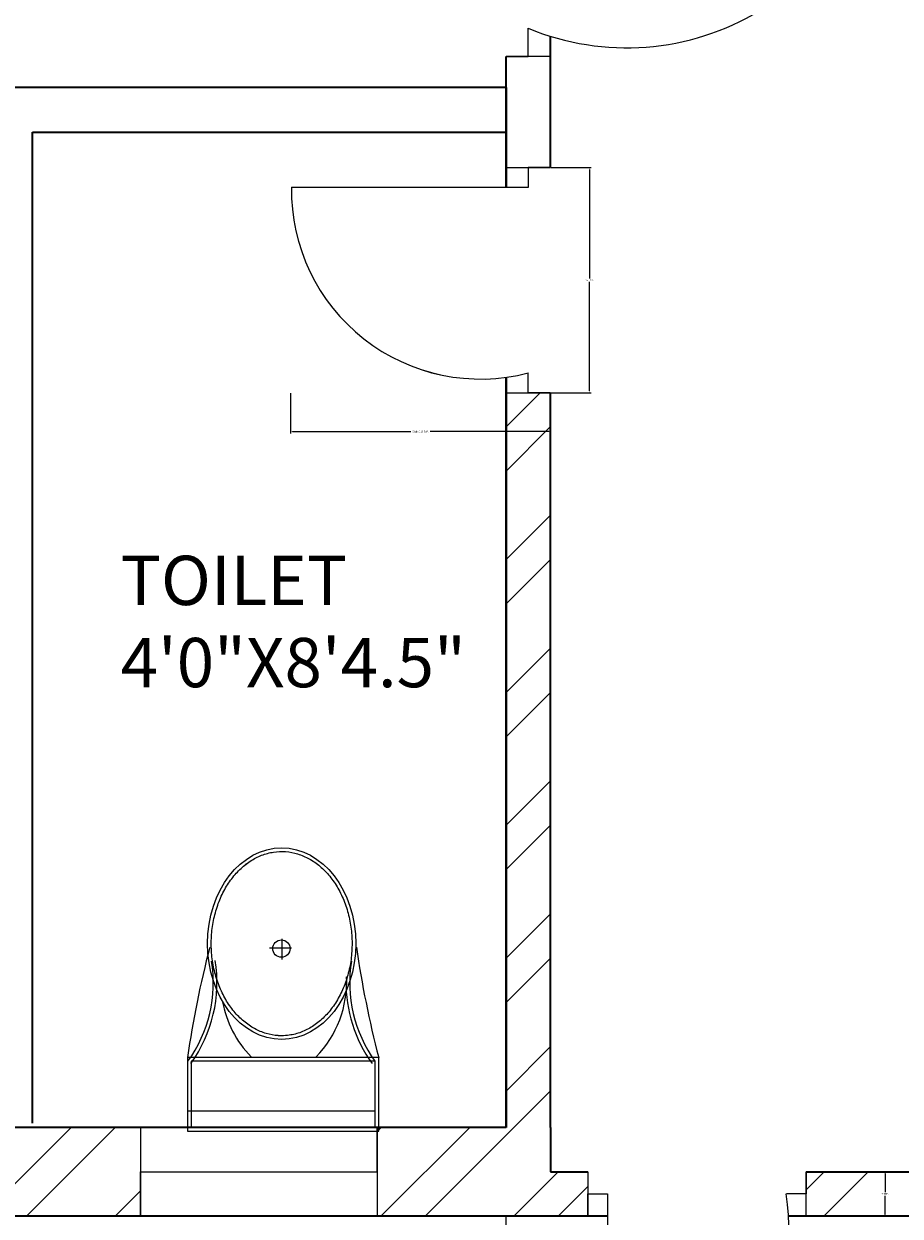
# Model space of a CAD drawing. Units: inches. Extents: x 2120 to 4013, y 1390 to 3019.
# Tile 10 of 59: x 2448 to 2537, y 1582 to 1702. Entities that reach past the tile are written whole.
import ezdxf

# ---------------------------------------------------------------- set-up
doc = ezdxf.new("R2010")
doc.units = ezdxf.units.IN
for name, color, linetype, lineweight in [('A-ANNO-DIMS', 2, 'Continuous', 18), ('A-AREA-IDEN', 7, 'Continuous', 18), ('A-DOOR', 3, 'Continuous', 18), ('A-FLOR-DECK', 7, 'Continuous', 25), ('A-FLOR-FIXT', 9, 'Continuous', 18), ('A-GLAZ', 4, 'Continuous', 18), ('A-WALL', 7, 'Continuous', 35), ('A-WALL-PATT', 252, 'Continuous', 13)]:
    doc.layers.add(name, color=color, linetype=linetype, lineweight=lineweight)
doc.styles.get("Standard").update_dxf_attribs({"font": 'arial.ttf'})
doc.dimstyles.get("Standard").update_dxf_attribs({"dimtxt": 0.18, "dimasz": 0.18, "dimexe": 0.18, "dimexo": 0.0625, "dimgap": 0.09, "dimtad": 0, "dimtih": 1, "dimtoh": 1, "dimdec": 4, "dimzin": 0, "dimdsep": 46, "dimtxsty": 'Standard', "dimcen": 0.09, "dimadec": 0, "dimazin": 0, "dimtfac": 1, "dimtdec": 4, "dimtofl": 0, "dimtmove": 0, "dimatfit": 3, "dimfxl": 1, "dimtolj": 1, "dimtzin": 0, "dimarcsym": 0})

# ---------------------------------------------------------------- blocks, each defined once
blk = doc.blocks.new('A$C31115884')
for p, q in [((257.5, 466.4), (257.5, 523.2)), ((283.1, 497.7), (223.4, 497.7)), ((0, 200), (0, 0)), ((520, 200), (0, 200)), ((520, 0), (520, 200)), ((10, 190), (10, 10)), ((510, 190), (10, 190)), ((510, 10), (510, 190)), ((510, 54.5), (0, 54.5)), ((10, 10), (510, 10)), ((0, 0), (520, 0))]:
    blk.add_line(p, q)
blk.add_circle((255.6, 496.4), 23.6)
for centre, radius, start, end in [((2777.7, -204.6), 2807, 165.4549, 171.7133), ((3237, 905), 2807, 188.2867, 194.5451), ((-294.5, 403.3), 364.7, 324.2091, 9.3499), ((-294.5, 403.3), 374.7, 324.2091, 9.3499), ((805.8, 403.3), 364.7, 170.6501, 215.7909), ((139.5, 406.2), 293.5, 315.8436, 2.6563), ((805.8, 403.3), 374.7, 179.2036, 215.7909), ((383.6, 406.2), 293.5, 190.2774, 224.1564)]:
    blk.add_arc(centre, radius, start, end)
blk.add_ellipse((256.2, 509.9), major_axis=(0, -260.7), ratio=0.772727)
blk.add_open_spline([(256.2, 259.2), (263.1, 259.2), (270, 259.7), (287.8, 262.3), (298.7, 265.1), (319.9, 273.1), (330.2, 278.4), (350.1, 291.1), (359.7, 298.7), (377.7, 315.9), (386.2, 325.5), (401.7, 346.6), (408.8, 358.1), (421.3, 382.5), (426.8, 395.5), (435.9, 422.4), (439.5, 436.4), (444.8, 465.1), (446.5, 479.7), (447.9, 509.2), (447.6, 524), (445, 553.3), (442.7, 567.8), (436.3, 596), (432.1, 609.7), (421.9, 636), (416, 648.6), (402.5, 672.1), (395, 683), (378.6, 703), (369.8, 712.1), (351.1, 728), (341.3, 734.8), (320.9, 746.2), (310.4, 750.7), (288.9, 757.3), (278, 759.4), (256, 761), (245, 760.6), (223.1, 757.2), (212.3, 754.3), (191.1, 746.1), (180.8, 740.7), (160.9, 727.8), (151.4, 720.1), (133.5, 702.7), (125.1, 693), (109.6, 671.7), (102.6, 660.2), (90.2, 635.7), (84.9, 622.7), (76, 595.6), (72.4, 581.6), (67.2, 552.9), (65.6, 538.2), (64.4, 508.8), (64.8, 494), (67.5, 464.7), (69.9, 450.2), (76.6, 422), (80.8, 408.3), (91.1, 382.2), (97.2, 369.7), (110.8, 346.3), (118.4, 335.4), (134.8, 315.6), (143.7, 306.7), (162.4, 290.9), (172.3, 284.2), (192.8, 273), (203.3, 268.6), (224.8, 262.2), (235.8, 260.2), (249.9, 259.3), (253, 259.2), (256.2, 259.2)], degree=3, knots=[0, 0, 0, 0, 0.110105, 0.110105, 0.285049, 0.285049, 0.459994, 0.459994, 0.634938, 0.634938, 0.809882, 0.809882, 0.984827, 0.984827, 1.159771, 1.159771, 1.334715, 1.334715, 1.50966, 1.50966, 1.684604, 1.684604, 1.859549, 1.859549, 2.034493, 2.034493, 2.209437, 2.209437, 2.384382, 2.384382, 2.559326, 2.559326, 2.73427, 2.73427, 2.909215, 2.909215, 3.084159, 3.084159, 3.259103, 3.259103, 3.434048, 3.434048, 3.608992, 3.608992, 3.783936, 3.783936, 3.958881, 3.958881, 4.133825, 4.133825, 4.30877, 4.30877, 4.483714, 4.483714, 4.658658, 4.658658, 4.833603, 4.833603, 5.008547, 5.008547, 5.183491, 5.183491, 5.358436, 5.358436, 5.53338, 5.53338, 5.708324, 5.708324, 5.883269, 5.883269, 6.058213, 6.058213, 6.233158, 6.233158, 6.283185, 6.283185, 6.283185, 6.283185])
blk = doc.blocks.new('DOOR-SWING-24IN-91p57DEG')
for p, q in [((0, 26.25), (0, 21.75)), ((22.12, 21.75), (22.12, 26.25)), ((22.12, 26.25), (22.12, 24)), ((0, 21.75), (0, 24)), ((0, 24), (2, 24)), ((2, 24), (2, 0)), ((22.12, 24), (20.12, 24))]:
    blk.add_line(p, q)
blk.add_arc((-0.62, 20.81), 20.98, 277.1643, 8.7385)
blk = doc.blocks.new('DOOR-SWING-24IN-105p55DEG')
for p, q in [((21.75, 22.82), (26.25, 22.82)), ((26.25, 22.82), (24, 22.82)), ((24, 22.82), (24, 20.82)), ((24, 20.82), (0, 20.82)), ((24, 0), (24, 2)), ((21.75, 0), (26.25, 0)), ((26.25, 0), (24, 0))]:
    blk.add_line(p, q)
blk.add_arc((19.15, 20.53), 19.15, 179.1207, 284.6739)
blk = doc.blocks.new('DOOR-SWING-36IN-107p00DEG')
for p, q in [((4.5, 26.58), (0, 26.58)), ((0, 26.58), (2.25, 26.58)), ((2.25, 26.58), (2.25, 24.58)), ((2.25, 24.58), (38.25, 24.58)), ((2.25, 0), (2.25, 2.87)), ((4.5, 0), (0, 0)), ((0, 0), (2.25, 0))]:
    blk.add_line(p, q)
blk.add_arc((12.22, 27.04), 26.15, 247.599, 354.5999)
blk = doc.blocks.new('WIN-PLAN-24IN-03')
for p, q in [((9, 24), (0, 24)), ((0, 24), (4.5, 24)), ((4.5, 24), (4.5, 0)), ((9, 0), (0, 0)), ((4.5, 0), (9, 0))]:
    blk.add_line(p, q)
blk = doc.blocks.new('*D137')
at = {"layer": 'A-ANNO-DIMS', "color": 0, "lineweight": -2, "transparency": 16777216}
for p, q in [((2474.89, 1664.96), (2474.89, 1660.89)), ((2501.23, 1664.96), (2501.23, 1660.89)), ((2475.07, 1661.07), (2487.07, 1661.07)), ((2501.05, 1661.07), (2489.05, 1661.07))]:
    blk.add_line(p, q, dxfattribs=at)
at = {"layer": 'A-ANNO-DIMS', "color": 0, "transparency": 16777216}
for points in [[(2475.07, 1661.1), (2475.07, 1661.04), (2474.89, 1661.07)], [(2501.05, 1661.1), (2501.05, 1661.04), (2501.23, 1661.07)]]:
    blk.add_solid(points, dxfattribs=at)
at = {"layer": 'Defpoints', "color": 0, "transparency": 16777216}
for p in [(2474.89, 1665.02), (2501.23, 1665.02), (2501.23, 1661.07)]:
    blk.add_point(p, dxfattribs=at)
at = {"layer": 'A-ANNO-DIMS', "color": 0, "transparency": 16777216, "insert": (2488.06, 1661.07), "char_height": 0.18, "attachment_point": 5}
blk.add_mtext('\\A1;SWING 26 TYP.', dxfattribs=at)
blk = doc.blocks.new('*D138')
at = {"layer": 'A-ANNO-DIMS', "color": 0, "lineweight": -2, "transparency": 16777216}
for p, q in [((2501.3, 1687.84), (2505.36, 1687.84)), ((2505.18, 1687.66), (2505.18, 1676.61)), ((2505.18, 1665.2), (2505.18, 1676.25)), ((2501.3, 1665.02), (2505.36, 1665.02))]:
    blk.add_line(p, q, dxfattribs=at)
at = {"layer": 'A-ANNO-DIMS', "color": 0, "transparency": 16777216}
for points in [[(2505.15, 1687.66), (2505.21, 1687.66), (2505.18, 1687.84)], [(2505.15, 1665.2), (2505.21, 1665.2), (2505.18, 1665.02)]]:
    blk.add_solid(points, dxfattribs=at)
at = {"layer": 'Defpoints', "color": 0, "transparency": 16777216}
for p in [(2501.23, 1687.84), (2505.18, 1687.84), (2501.23, 1665.02)]:
    blk.add_point(p, dxfattribs=at)
at = {"layer": 'A-ANNO-DIMS', "color": 0, "transparency": 16777216, "insert": (2505.18, 1676.43), "char_height": 0.18, "attachment_point": 5}
blk.add_mtext('\\A1;23 TYP.', dxfattribs=at)
blk = doc.blocks.new('*D192')
at = {"layer": 'A-ANNO-DIMS', "color": 0, "lineweight": -2, "transparency": 16777216}
for p, q in [((2544.07, 1586.03), (2534.96, 1586.03)), ((2535.14, 1585.85), (2535.14, 1583.96)), ((2535.14, 1581.71), (2535.14, 1583.6)), ((2544.07, 1581.53), (2534.96, 1581.53))]:
    blk.add_line(p, q, dxfattribs=at)
at = {"layer": 'A-ANNO-DIMS', "color": 0, "transparency": 16777216}
for points in [[(2535.11, 1585.85), (2535.17, 1585.85), (2535.14, 1586.03)], [(2535.11, 1581.71), (2535.17, 1581.71), (2535.14, 1581.53)]]:
    blk.add_solid(points, dxfattribs=at)
at = {"layer": 'Defpoints', "color": 0, "transparency": 16777216}
for p in [(2535.14, 1586.03), (2544.14, 1586.03), (2544.14, 1581.53)]:
    blk.add_point(p, dxfattribs=at)
at = {"layer": 'A-ANNO-DIMS', "color": 0, "transparency": 16777216, "insert": (2535.14, 1583.78), "char_height": 0.18, "attachment_point": 5}
blk.add_mtext('\\A1;5 TYP.', dxfattribs=at)

msp = doc.modelspace()

# ---------------------------------------------------------------- hatches: boundary and pattern name
at = {"layer": 'A-WALL-PATT'}
h = msp.add_hatch(dxfattribs=at)
h.set_pattern_fill('ANSI32', color=256)
h.paths.add_polyline_path([(2271.7331, 2343.531), (2283.3788, 2343.531), (2283.3788, 2348.031), (2283.3788, 2352.5306), (2262.7331, 2352.5306), (2262.7331, 2182.638), (2267.2331, 2182.638), (2271.7331, 2182.638), (2271.7331, 2219.031), (2391.7331, 2219.031), (2391.7331, 2214.189), (2393.9831, 2214.189), (2396.2331, 2214.189), (2396.2331, 2219.031), (2420.2331, 2219.031), (2420.2331, 2225.7535), (2417.2197, 2225.7535), (2415.7331, 2225.7535), (2415.7331, 2223.5306), (2271.7331, 2223.5306)])
h.paths.add_polyline_path([(2380.0942, 2352.5306), (2343.3788, 2352.5306), (2343.3788, 2343.531), (2363.2331, 2343.531), (2363.2331, 2288.8489), (2365.4831, 2288.8489), (2367.7331, 2288.8489), (2367.7331, 2343.531), (2380.0942, 2343.531)], flags=17)
h.paths.add_polyline_path([(2432.4339, 2352.5306), (2404.0943, 2352.5306), (2404.0943, 2343.531), (2415.7331, 2343.531), (2415.7331, 2264.0306), (2367.7331, 2264.0306), (2367.7331, 2266.4872), (2363.2331, 2266.4872), (2363.2331, 2259.531), (2367.7331, 2259.531), (2415.7331, 2259.531), (2415.7331, 2255.0658), (2420.2331, 2255.0658), (2420.2331, 2259.531), (2424.5717, 2259.531), (2424.5717, 2261.781), (2424.5717, 2264.0306), (2420.2331, 2264.0306), (2420.2331, 2343.531), (2432.4339, 2343.531)])
h.paths.add_polyline_path([(2508.9115, 2352.5306), (2456.4339, 2352.5306), (2456.4339, 2343.531), (2468.2331, 2343.531), (2468.2331, 2264.0306), (2448.0487, 2264.0306), (2448.0487, 2259.531), (2468.2331, 2259.531), (2468.2331, 2255.5496), (2472.7331, 2255.5496), (2472.7331, 2343.531), (2508.9115, 2343.531)])
h.paths.add_polyline_path([(2637.7331, 2352.5306), (2544.9116, 2352.5306), (2544.9116, 2343.531), (2589.7331, 2343.531), (2633.2331, 2343.531), (2637.7331, 2343.531)])
h.paths.add_polyline_path([(2594.2331, 2343.5306), (2589.7331, 2343.5306), (2589.7331, 2259.5306), (2589.7331, 2252.4915), (2591.9831, 2252.4915), (2594.2331, 2252.4915)])
h.paths.add_polyline_path([(2637.7331, 2223.5306), (2594.2331, 2223.5306), (2594.2331, 2230.1988), (2591.9831, 2230.1988), (2589.7331, 2230.1988), (2589.7331, 2223.5306), (2472.7331, 2223.5306), (2468.2331, 2223.5306), (2468.2331, 2219.031), (2628.7331, 2219.031), (2628.7331, 2138.031), (2637.7331, 2138.031)])
h.paths.add_polyline_path([(3822.6535, 2458.4402), (3874.9468, 2458.4402), (3874.9468, 2476.9866), (3822.6535, 2476.9866)], flags=9)
h.paths.add_polyline_path([(3834.6921, 2781.8174), (3935.9206, 2781.8174), (3935.9206, 2800.3638), (3834.6921, 2800.3638)], flags=9)
h.paths.add_polyline_path([(3832.2843, 2837.9683), (3884.5776, 2837.9683), (3884.5776, 2856.5146), (3832.2843, 2856.5146)], flags=9)
h.paths.add_polyline_path([(3830.9388, 2861.4782), (3956.8958, 2861.4782), (3956.8958, 2880.0245), (3830.9388, 2880.0245)], flags=9)
h.paths.add_polyline_path([(3870.6966, 2352.5752), (3887.9272, 2352.5752), (3887.9272, 2377.3037), (3870.6966, 2377.3037)], flags=9)
h.paths.add_polyline_path([(3289.2701, 2413.161), (3435.2223, 2413.161), (3435.2223, 2450.2538), (3289.2701, 2450.2538)], flags=9)
h.paths.add_polyline_path([(2487.6944, 2414.3601), (2637.8335, 2414.3601), (2637.8335, 2451.4528), (2487.6944, 2451.4528)], flags=9)
h.paths.add_polyline_path([(2567.3724, 1457.9199), (2815.296, 1457.9199), (2815.296, 1495.0127), (2567.3724, 1495.0127)], flags=9)
h.paths.add_polyline_path([(2655.3825, 2093.2363), (2685.9555, 2093.2363), (2685.9555, 2111.8937), (2655.3825, 2111.8937)], flags=9)
h.paths.add_polyline_path([(2543.9218, 1550.6671), (2587.8406, 1550.6671), (2587.8406, 1569.3244), (2543.9218, 1569.3244)], flags=9)
h.paths.add_polyline_path([(2905.1384, 1543.8113), (2949.0572, 1543.8113), (2949.0572, 1562.4686), (2905.1384, 1562.4686)], flags=9)
h.paths.add_polyline_path([(2736.4118, 1702.4736), (2784.2153, 1702.4736), (2784.2153, 1721.1309), (2736.4118, 1721.1309)], flags=9)
h.paths.add_polyline_path([(2912.8666, 1710.4168), (2951.707, 1710.4168), (2951.707, 1729.0741), (2912.8666, 1729.0741)], flags=9)
h.paths.add_polyline_path([(2923.5785, 1763.5038), (2959.7279, 1763.5038), (2959.7279, 1782.1611), (2923.5785, 1782.1611)], flags=9)
h.paths.add_polyline_path([(2925.2114, 1809.6137), (2967.1861, 1809.6137), (2967.1861, 1828.271), (2925.2114, 1828.271)], flags=9)
h.paths.add_polyline_path([(2996.2711, 1878.9003), (2996.2711, 1913.109), (2977.6138, 1913.109), (2977.6138, 1878.9003)], flags=9)
h.paths.add_polyline_path([(2883.0859, 1895.7192), (2927.1855, 1895.7192), (2927.1855, 1914.3766), (2883.0859, 1914.3766)], flags=9)
h.paths.add_polyline_path([(2787.3924, 1810.8013), (2841.0213, 1810.8013), (2841.0213, 1829.4587), (2787.3924, 1829.4587)], flags=9)
h.paths.add_polyline_path([(2775.6399, 2101.7395), (2829.2689, 2101.7395), (2829.2689, 2120.3968), (2775.6399, 2120.3968)], flags=9)
h.paths.add_polyline_path([(2913.0263, 2075.817), (2951.8667, 2075.817), (2951.8667, 2094.4744), (2913.0263, 2094.4744)], flags=9)
h.paths.add_polyline_path([(2929.966, 2133.3669), (2966.1154, 2133.3669), (2966.1154, 2152.0243), (2929.966, 2152.0243)], flags=9)
h.paths.add_polyline_path([(2932.7502, 2182.6088), (2968.8996, 2182.6088), (2968.8996, 2201.2662), (2932.7502, 2201.2662)], flags=9)
h.paths.add_polyline_path([(2996.0681, 2266.3173), (2996.0681, 2300.5261), (2977.4108, 2300.5261), (2977.4108, 2266.3173)], flags=9)
h.paths.add_polyline_path([(2885.1039, 2279.2186), (2929.2035, 2279.2186), (2929.2035, 2297.8759), (2885.1039, 2297.8759)], flags=9)
h.paths.add_polyline_path([(2735.7042, 2218.3197), (2783.5078, 2218.3197), (2783.5078, 2236.9771), (2735.7042, 2236.9771)], flags=9)
h.paths.add_polyline_path([(2635.6049, 2044.0085), (2648.9678, 2044.0085), (2648.9678, 2054.312), (2635.6049, 2054.312)], flags=9)
h.paths.add_polyline_path([(2714.0148, 1923.0473), (2727.3777, 1923.0473), (2727.3777, 1933.3508), (2714.0148, 1933.3508)], flags=9)
h.paths.add_polyline_path([(2709.0345, 1988.1628), (2722.3974, 1988.1628), (2722.3974, 1998.4663), (2709.0345, 1998.4663)], flags=9)
h.paths.add_polyline_path([(2592.8935, 1962.1763), (2606.2564, 1962.1763), (2606.2564, 1972.4799), (2592.8935, 1972.4799)], flags=9)
h.paths.add_polyline_path([(2618.3996, 1985.9724), (2644.1942, 1985.9724), (2644.1942, 1996.2759), (2618.3996, 1996.2759)], flags=9)
h.paths.add_polyline_path([(2601.279, 1920.5869), (2614.6419, 1920.5869), (2614.6419, 1930.8904), (2601.279, 1930.8904)], flags=9)
h.paths.add_polyline_path([(2692.3278, 1932.7645), (2704.5311, 1932.7645), (2704.5311, 1943.0681), (2692.3278, 1943.0681)], flags=9)
h.paths.add_polyline_path([(2311.122, 1672.7318), (2355.0408, 1672.7318), (2355.0408, 1691.3892), (2311.122, 1691.3892)], flags=9)
h.paths.add_polyline_path([(2456.2551, 1632.3198), (2492.4796, 1632.3198), (2492.4796, 1650.9772), (2456.2551, 1650.9772)], flags=9)
h.paths.add_polyline_path([(2401.0766, 1631.4793), (2437.301, 1631.4793), (2437.301, 1650.1367), (2401.0766, 1650.1367)], flags=9)
h.paths.add_polyline_path([(2546.7054, 1700.9235), (2594.509, 1700.9235), (2594.509, 1719.5809), (2546.7054, 1719.5809)], flags=9)
h.paths.add_polyline_path([(2445.4866, 1766.9937), (2497.5261, 1766.9937), (2497.5261, 1785.651), (2445.4866, 1785.651)], flags=9)
h.paths.add_polyline_path([(2287.9992, 1739.7675), (2326.8396, 1739.7675), (2326.8396, 1758.4248), (2287.9992, 1758.4248)], flags=9)
h.paths.add_polyline_path([(2458.5279, 1924.7607), (2510.5675, 1924.7607), (2510.5675, 1943.4181), (2458.5279, 1943.4181)], flags=9)
h.paths.add_polyline_path([(2309.2811, 1902.7642), (2345.4305, 1902.7642), (2345.4305, 1921.4215), (2309.2811, 1921.4215)], flags=9)
h.paths.add_polyline_path([(2490.7554, 2018.9392), (2530.7896, 2018.9392), (2530.7896, 2037.5965), (2490.7554, 2037.5965)], flags=9)
h.paths.add_polyline_path([(2402.143, 2024.7393), (2438.5414, 2024.7393), (2438.5414, 2043.3966), (2402.143, 2043.3966)], flags=9)
h.paths.add_polyline_path([(2287.856, 1931.7926), (2326.6964, 1931.7926), (2326.6964, 1950.4499), (2287.856, 1950.4499)], flags=9)
h.paths.add_polyline_path([(2281.7979, 2193.5771), (2320.6383, 2193.5771), (2320.6383, 2212.2344), (2281.7979, 2212.2344)], flags=25)
h.paths.add_polyline_path([(2484.0754, 2093.892), (2536.115, 2093.892), (2536.115, 2112.5494), (2484.0754, 2112.5494)], flags=9)
h.paths.add_polyline_path([(2624.7948, 2281.8639), (2624.7948, 2311.4137), (2606.1375, 2311.4137), (2606.1375, 2281.8639)], flags=9)
h.paths.add_polyline_path([(2507.5036, 2290.3639), (2541.934, 2290.3639), (2541.934, 2309.0212), (2507.5036, 2309.0212)], flags=9)
h.paths.add_polyline_path([(2423.1076, 2285.2202), (2459.332, 2285.2202), (2459.332, 2303.8776), (2423.1076, 2303.8776)], flags=9)
h.paths.add_polyline_path([(2374.5467, 2289.6272), (2410.7711, 2289.6272), (2410.7711, 2308.2846), (2374.5467, 2308.2846)], flags=25)
h.paths.add_polyline_path([(2277.4907, 2227.5651), (2316.3311, 2227.5651), (2316.3311, 2246.2224), (2277.4907, 2246.2224)], flags=25)
h.paths.add_polyline_path([(2655.3825, 2093.2367), (2685.9555, 2093.2367), (2685.9555, 2111.894), (2655.3825, 2111.894)], flags=9)
h.paths.add_polyline_path([(2543.9217, 1550.6674), (2587.8406, 1550.6674), (2587.8406, 1569.3247), (2543.9217, 1569.3247)], flags=9)
h.paths.add_polyline_path([(2905.1384, 1543.8116), (2949.0572, 1543.8116), (2949.0572, 1562.4689), (2905.1384, 1562.4689)], flags=9)
h.paths.add_polyline_path([(2736.4118, 1702.4739), (2784.2153, 1702.4739), (2784.2153, 1721.1312), (2736.4118, 1721.1312)], flags=9)
h.paths.add_polyline_path([(2912.8666, 1710.4171), (2951.707, 1710.4171), (2951.707, 1729.0744), (2912.8666, 1729.0744)], flags=9)
h.paths.add_polyline_path([(2923.5785, 1763.5041), (2959.7279, 1763.5041), (2959.7279, 1782.1614), (2923.5785, 1782.1614)], flags=9)
h.paths.add_polyline_path([(2925.2114, 1809.614), (2967.1861, 1809.614), (2967.1861, 1828.2713), (2925.2114, 1828.2713)], flags=9)
h.paths.add_polyline_path([(2996.2711, 1878.9006), (2996.2711, 1913.1094), (2977.6137, 1913.1094), (2977.6137, 1878.9006)], flags=9)
h.paths.add_polyline_path([(2883.0859, 1895.7195), (2927.1855, 1895.7195), (2927.1855, 1914.3769), (2883.0859, 1914.3769)], flags=9)
h.paths.add_polyline_path([(2787.3924, 1810.8016), (2841.0213, 1810.8016), (2841.0213, 1829.459), (2787.3924, 1829.459)], flags=9)
h.paths.add_polyline_path([(2775.6399, 2101.7398), (2829.2688, 2101.7398), (2829.2688, 2120.3971), (2775.6399, 2120.3971)], flags=9)
h.paths.add_polyline_path([(2913.0263, 2075.8173), (2951.8667, 2075.8173), (2951.8667, 2094.4747), (2913.0263, 2094.4747)], flags=9)
h.paths.add_polyline_path([(2929.966, 2133.3672), (2966.1154, 2133.3672), (2966.1154, 2152.0246), (2929.966, 2152.0246)], flags=9)
h.paths.add_polyline_path([(2932.7502, 2182.6091), (2968.8996, 2182.6091), (2968.8996, 2201.2665), (2932.7502, 2201.2665)], flags=9)
h.paths.add_polyline_path([(2996.0681, 2266.3176), (2996.0681, 2300.5264), (2977.4108, 2300.5264), (2977.4108, 2266.3176)], flags=9)
h.paths.add_polyline_path([(2885.1039, 2279.2189), (2929.2035, 2279.2189), (2929.2035, 2297.8762), (2885.1039, 2297.8762)], flags=9)
h.paths.add_polyline_path([(2735.7042, 2218.32), (2783.5078, 2218.32), (2783.5078, 2236.9774), (2735.7042, 2236.9774)], flags=9)
h.paths.add_polyline_path([(2635.6048, 2044.0088), (2648.9677, 2044.0088), (2648.9677, 2054.3123), (2635.6048, 2054.3123)], flags=9)
h.paths.add_polyline_path([(2714.0148, 1923.0476), (2727.3777, 1923.0476), (2727.3777, 1933.3511), (2714.0148, 1933.3511)], flags=9)
h.paths.add_polyline_path([(2709.0345, 1988.1631), (2722.3974, 1988.1631), (2722.3974, 1998.4666), (2709.0345, 1998.4666)], flags=9)
h.paths.add_polyline_path([(2592.8935, 1962.1766), (2606.2564, 1962.1766), (2606.2564, 1972.4802), (2592.8935, 1972.4802)], flags=9)
h.paths.add_polyline_path([(2618.3995, 1985.9727), (2644.1942, 1985.9727), (2644.1942, 1996.2762), (2618.3995, 1996.2762)], flags=9)
h.paths.add_polyline_path([(2601.279, 1920.5872), (2614.6419, 1920.5872), (2614.6419, 1930.8908), (2601.279, 1930.8908)], flags=9)
h.paths.add_polyline_path([(2692.3278, 1932.7648), (2704.5311, 1932.7648), (2704.5311, 1943.0684), (2692.3278, 1943.0684)], flags=9)
h.paths.add_polyline_path([(2311.122, 1672.7321), (2355.0408, 1672.7321), (2355.0408, 1691.3895), (2311.122, 1691.3895)], flags=9)
h.paths.add_polyline_path([(2456.2551, 1632.3201), (2492.4795, 1632.3201), (2492.4795, 1650.9775), (2456.2551, 1650.9775)], flags=9)
h.paths.add_polyline_path([(2401.0766, 1631.4796), (2437.301, 1631.4796), (2437.301, 1650.137), (2401.0766, 1650.137)], flags=9)
h.paths.add_polyline_path([(2546.7054, 1700.9238), (2594.509, 1700.9238), (2594.509, 1719.5812), (2546.7054, 1719.5812)], flags=9)
h.paths.add_polyline_path([(2445.4866, 1766.994), (2497.5261, 1766.994), (2497.5261, 1785.6513), (2445.4866, 1785.6513)], flags=9)
h.paths.add_polyline_path([(2287.9992, 1739.7678), (2326.8396, 1739.7678), (2326.8396, 1758.4251), (2287.9992, 1758.4251)], flags=9)
h.paths.add_polyline_path([(2458.5279, 1924.7611), (2510.5675, 1924.7611), (2510.5675, 1943.4184), (2458.5279, 1943.4184)], flags=9)
h.paths.add_polyline_path([(2309.2811, 1902.7645), (2345.4305, 1902.7645), (2345.4305, 1921.4218), (2309.2811, 1921.4218)], flags=9)
h.paths.add_polyline_path([(2490.7554, 2018.9395), (2530.7895, 2018.9395), (2530.7895, 2037.5968), (2490.7554, 2037.5968)], flags=9)
h.paths.add_polyline_path([(2402.143, 2024.7396), (2438.5413, 2024.7396), (2438.5413, 2043.3969), (2402.143, 2043.3969)], flags=9)
h.paths.add_polyline_path([(2287.856, 1931.7929), (2326.6964, 1931.7929), (2326.6964, 1950.4502), (2287.856, 1950.4502)], flags=9)
h.paths.add_polyline_path([(2281.7979, 2193.5774), (2320.6383, 2193.5774), (2320.6383, 2212.2347), (2281.7979, 2212.2347)], flags=25)
h.paths.add_polyline_path([(2484.0754, 2093.8924), (2536.115, 2093.8924), (2536.115, 2112.5497), (2484.0754, 2112.5497)], flags=9)
h.paths.add_polyline_path([(2624.7948, 2281.8642), (2624.7948, 2311.414), (2606.1374, 2311.414), (2606.1374, 2281.8642)], flags=9)
h.paths.add_polyline_path([(2507.5035, 2290.3642), (2541.934, 2290.3642), (2541.934, 2309.0215), (2507.5035, 2309.0215)], flags=9)
h.paths.add_polyline_path([(2423.1075, 2285.2205), (2459.332, 2285.2205), (2459.332, 2303.8779), (2423.1075, 2303.8779)], flags=9)
h.paths.add_polyline_path([(2374.5467, 2289.6275), (2410.7711, 2289.6275), (2410.7711, 2308.2849), (2374.5467, 2308.2849)], flags=25)
h.paths.add_polyline_path([(2277.4907, 2227.5654), (2316.3311, 2227.5654), (2316.3311, 2246.2227), (2277.4907, 2246.2227)], flags=25)
h = msp.add_hatch(dxfattribs=at)
h.set_pattern_fill('ANSI32', color=256)
h.paths.add_polyline_path([(2271.7331, 1980.389), (2262.7331, 1980.389), (2262.7331, 1912.8434), (2267.2331, 1912.8434), (2271.7331, 1912.8434), (2271.7331, 1922.531), (2351.2331, 1922.531), (2351.2331, 1901.4728), (2355.7331, 1901.4728), (2355.7331, 1922.531), (2357.9815, 1922.531), (2357.9815, 1926.5306), (2271.7331, 1926.5306)])
h.paths.add_polyline_path([(2589.2331, 1949.1622), (2584.7331, 1949.1622), (2580.2331, 1949.1622), (2580.2331, 1874.5306), (2355.7331, 1874.5306), (2355.7331, 1880.1922), (2351.2331, 1880.1922), (2351.2331, 1874.5306), (2271.7331, 1874.5306), (2271.7331, 1888.8431), (2262.7331, 1888.8431), (2262.7331, 1842.2909), (2267.2331, 1842.2909), (2271.7331, 1842.2909), (2271.7331, 1865.531), (2415.7331, 1865.531), (2415.7331, 1779.7286), (2420.2331, 1779.7286), (2420.2331, 1865.531), (2589.2331, 1865.531)])
h.paths.add_polyline_path([(2271.7331, 1782.2906), (2262.7331, 1782.2906), (2262.7331, 1711.4639), (2267.2331, 1711.4639), (2271.7331, 1711.4639), (2271.7331, 1738.031), (2420.2331, 1738.031), (2420.2331, 1742.531), (2420.2331, 1747.3376), (2417.9831, 1747.3376), (2415.7331, 1747.3376), (2415.7331, 1742.5306), (2271.7331, 1742.5306)])
h.paths.add_polyline_path([(2271.7331, 1627.031), (2362.3957, 1627.031), (2362.3957, 1629.281), (2362.3957, 1631.5306), (2271.7331, 1631.5306), (2271.7331, 1675.4636), (2262.7331, 1675.4636), (2262.7331, 1581.531), (2405.3032, 1581.531), (2405.3032, 1586.031), (2405.3032, 1590.5306), (2396.2331, 1590.5306), (2396.2331, 1691.4513), (2418.7206, 1691.4513), (2418.7206, 1695.951), (2396.2331, 1695.951), (2391.7331, 1695.951), (2391.7331, 1631.5306), (2386.7425, 1631.5306), (2386.7425, 1629.2806), (2386.7425, 1627.031), (2391.7331, 1627.031), (2391.7331, 1586.1709), (2271.7331, 1586.1709)])
h.paths.add_polyline_path([(2459.6703, 1590.5306), (2429.3032, 1590.5306), (2429.3032, 1581.531), (2459.6703, 1581.531), (2459.6703, 1586.031)])
h.paths.add_polyline_path([(2501.2331, 1590.531), (2501.2331, 1665.0195), (2498.9831, 1665.0195), (2496.7331, 1665.0195), (2496.7331, 1590.5306), (2483.8201, 1590.5306), (2483.8201, 1590.1579), (2483.6704, 1590.1579), (2483.6704, 1581.531), (2505.0196, 1581.531), (2505.0196, 1583.781), (2505.0196, 1586.0306), (2501.2331, 1586.0306)])
h.paths.add_polyline_path([(2544.1361, 1583.781), (2544.1361, 1586.0306), (2527.1368, 1586.0306), (2527.1368, 1583.7806), (2527.1368, 1581.531), (2544.1361, 1581.531)])
h.paths.add_polyline_path([(3822.6535, 2458.4402), (3874.9468, 2458.4402), (3874.9468, 2476.9866), (3822.6535, 2476.9866)], flags=9)
h.paths.add_polyline_path([(3834.6921, 2781.8174), (3935.9206, 2781.8174), (3935.9206, 2800.3638), (3834.6921, 2800.3638)], flags=9)
h.paths.add_polyline_path([(3832.2843, 2837.9683), (3884.5776, 2837.9683), (3884.5776, 2856.5146), (3832.2843, 2856.5146)], flags=9)
h.paths.add_polyline_path([(3830.9388, 2861.4782), (3956.8958, 2861.4782), (3956.8958, 2880.0245), (3830.9388, 2880.0245)], flags=9)
h.paths.add_polyline_path([(3870.6966, 2352.5752), (3887.9272, 2352.5752), (3887.9272, 2377.3037), (3870.6966, 2377.3037)], flags=9)
h.paths.add_polyline_path([(3289.2701, 2413.161), (3435.2223, 2413.161), (3435.2223, 2450.2538), (3289.2701, 2450.2538)], flags=9)
h.paths.add_polyline_path([(2487.6944, 2414.3601), (2637.8335, 2414.3601), (2637.8335, 2451.4528), (2487.6944, 2451.4528)], flags=9)
h.paths.add_polyline_path([(2567.3724, 1457.9199), (2815.296, 1457.9199), (2815.296, 1495.0127), (2567.3724, 1495.0127)], flags=9)
h.paths.add_polyline_path([(2655.3825, 2093.2363), (2685.9555, 2093.2363), (2685.9555, 2111.8937), (2655.3825, 2111.8937)], flags=9)
h.paths.add_polyline_path([(2543.9218, 1550.6671), (2587.8406, 1550.6671), (2587.8406, 1569.3244), (2543.9218, 1569.3244)], flags=9)
h.paths.add_polyline_path([(2905.1384, 1543.8113), (2949.0572, 1543.8113), (2949.0572, 1562.4686), (2905.1384, 1562.4686)], flags=9)
h.paths.add_polyline_path([(2736.4118, 1702.4736), (2784.2153, 1702.4736), (2784.2153, 1721.1309), (2736.4118, 1721.1309)], flags=9)
h.paths.add_polyline_path([(2912.8666, 1710.4168), (2951.707, 1710.4168), (2951.707, 1729.0741), (2912.8666, 1729.0741)], flags=9)
h.paths.add_polyline_path([(2923.5785, 1763.5038), (2959.7279, 1763.5038), (2959.7279, 1782.1611), (2923.5785, 1782.1611)], flags=9)
h.paths.add_polyline_path([(2925.2114, 1809.6137), (2967.1861, 1809.6137), (2967.1861, 1828.271), (2925.2114, 1828.271)], flags=9)
h.paths.add_polyline_path([(2996.2711, 1878.9003), (2996.2711, 1913.109), (2977.6138, 1913.109), (2977.6138, 1878.9003)], flags=9)
h.paths.add_polyline_path([(2883.0859, 1895.7192), (2927.1855, 1895.7192), (2927.1855, 1914.3766), (2883.0859, 1914.3766)], flags=9)
h.paths.add_polyline_path([(2787.3924, 1810.8013), (2841.0213, 1810.8013), (2841.0213, 1829.4587), (2787.3924, 1829.4587)], flags=9)
h.paths.add_polyline_path([(2775.6399, 2101.7395), (2829.2689, 2101.7395), (2829.2689, 2120.3968), (2775.6399, 2120.3968)], flags=9)
h.paths.add_polyline_path([(2913.0263, 2075.817), (2951.8667, 2075.817), (2951.8667, 2094.4744), (2913.0263, 2094.4744)], flags=9)
h.paths.add_polyline_path([(2929.966, 2133.3669), (2966.1154, 2133.3669), (2966.1154, 2152.0243), (2929.966, 2152.0243)], flags=9)
h.paths.add_polyline_path([(2932.7502, 2182.6088), (2968.8996, 2182.6088), (2968.8996, 2201.2662), (2932.7502, 2201.2662)], flags=9)
h.paths.add_polyline_path([(2996.0681, 2266.3173), (2996.0681, 2300.5261), (2977.4108, 2300.5261), (2977.4108, 2266.3173)], flags=9)
h.paths.add_polyline_path([(2885.1039, 2279.2186), (2929.2035, 2279.2186), (2929.2035, 2297.8759), (2885.1039, 2297.8759)], flags=9)
h.paths.add_polyline_path([(2735.7042, 2218.3197), (2783.5078, 2218.3197), (2783.5078, 2236.9771), (2735.7042, 2236.9771)], flags=9)
h.paths.add_polyline_path([(2635.6049, 2044.0085), (2648.9678, 2044.0085), (2648.9678, 2054.312), (2635.6049, 2054.312)], flags=9)
h.paths.add_polyline_path([(2714.0148, 1923.0473), (2727.3777, 1923.0473), (2727.3777, 1933.3508), (2714.0148, 1933.3508)], flags=9)
h.paths.add_polyline_path([(2709.0345, 1988.1628), (2722.3974, 1988.1628), (2722.3974, 1998.4663), (2709.0345, 1998.4663)], flags=9)
h.paths.add_polyline_path([(2592.8935, 1962.1763), (2606.2564, 1962.1763), (2606.2564, 1972.4799), (2592.8935, 1972.4799)], flags=9)
h.paths.add_polyline_path([(2618.3996, 1985.9724), (2644.1942, 1985.9724), (2644.1942, 1996.2759), (2618.3996, 1996.2759)], flags=9)
h.paths.add_polyline_path([(2601.279, 1920.5869), (2614.6419, 1920.5869), (2614.6419, 1930.8904), (2601.279, 1930.8904)], flags=9)
h.paths.add_polyline_path([(2692.3278, 1932.7645), (2704.5311, 1932.7645), (2704.5311, 1943.0681), (2692.3278, 1943.0681)], flags=9)
h.paths.add_polyline_path([(2311.122, 1672.7318), (2355.0408, 1672.7318), (2355.0408, 1691.3892), (2311.122, 1691.3892)], flags=25)
h.paths.add_polyline_path([(2456.2551, 1632.3198), (2492.4796, 1632.3198), (2492.4796, 1650.9772), (2456.2551, 1650.9772)], flags=9)
h.paths.add_polyline_path([(2401.0766, 1631.4793), (2437.301, 1631.4793), (2437.301, 1650.1367), (2401.0766, 1650.1367)], flags=9)
h.paths.add_polyline_path([(2546.7054, 1700.9235), (2594.509, 1700.9235), (2594.509, 1719.5809), (2546.7054, 1719.5809)], flags=9)
h.paths.add_polyline_path([(2445.4866, 1766.9937), (2497.5261, 1766.9937), (2497.5261, 1785.651), (2445.4866, 1785.651)], flags=9)
h.paths.add_polyline_path([(2287.9992, 1739.7675), (2326.8396, 1739.7675), (2326.8396, 1758.4248), (2287.9992, 1758.4248)], flags=24)
h.paths.add_polyline_path([(2458.5279, 1924.7607), (2510.5675, 1924.7607), (2510.5675, 1943.4181), (2458.5279, 1943.4181)], flags=25)
h.paths.add_polyline_path([(2309.2811, 1902.7642), (2345.4305, 1902.7642), (2345.4305, 1921.4215), (2309.2811, 1921.4215)], flags=25)
h.paths.add_polyline_path([(2490.7554, 2018.9392), (2530.7896, 2018.9392), (2530.7896, 2037.5965), (2490.7554, 2037.5965)], flags=9)
h.paths.add_polyline_path([(2402.143, 2024.7393), (2438.5414, 2024.7393), (2438.5414, 2043.3966), (2402.143, 2043.3966)], flags=9)
h.paths.add_polyline_path([(2287.856, 1931.7926), (2326.6964, 1931.7926), (2326.6964, 1950.4499), (2287.856, 1950.4499)], flags=25)
h.paths.add_polyline_path([(2281.7979, 2193.5771), (2320.6383, 2193.5771), (2320.6383, 2212.2344), (2281.7979, 2212.2344)], flags=9)
h.paths.add_polyline_path([(2484.0754, 2093.892), (2536.115, 2093.892), (2536.115, 2112.5494), (2484.0754, 2112.5494)], flags=9)
h.paths.add_polyline_path([(2624.7948, 2281.8639), (2624.7948, 2311.4137), (2606.1375, 2311.4137), (2606.1375, 2281.8639)], flags=9)
h.paths.add_polyline_path([(2507.5036, 2290.3639), (2541.934, 2290.3639), (2541.934, 2309.0212), (2507.5036, 2309.0212)], flags=9)
h.paths.add_polyline_path([(2423.1076, 2285.2202), (2459.332, 2285.2202), (2459.332, 2303.8776), (2423.1076, 2303.8776)], flags=9)
h.paths.add_polyline_path([(2374.5467, 2289.6272), (2410.7711, 2289.6272), (2410.7711, 2308.2846), (2374.5467, 2308.2846)], flags=9)
h.paths.add_polyline_path([(2277.4907, 2227.5651), (2316.3311, 2227.5651), (2316.3311, 2246.2224), (2277.4907, 2246.2224)], flags=9)
h.paths.add_polyline_path([(2655.3825, 2093.2367), (2685.9555, 2093.2367), (2685.9555, 2111.894), (2655.3825, 2111.894)], flags=9)
h.paths.add_polyline_path([(2543.9217, 1550.6674), (2587.8406, 1550.6674), (2587.8406, 1569.3247), (2543.9217, 1569.3247)], flags=9)
h.paths.add_polyline_path([(2905.1384, 1543.8116), (2949.0572, 1543.8116), (2949.0572, 1562.4689), (2905.1384, 1562.4689)], flags=9)
h.paths.add_polyline_path([(2736.4118, 1702.4739), (2784.2153, 1702.4739), (2784.2153, 1721.1312), (2736.4118, 1721.1312)], flags=9)
h.paths.add_polyline_path([(2912.8666, 1710.4171), (2951.707, 1710.4171), (2951.707, 1729.0744), (2912.8666, 1729.0744)], flags=9)
h.paths.add_polyline_path([(2923.5785, 1763.5041), (2959.7279, 1763.5041), (2959.7279, 1782.1614), (2923.5785, 1782.1614)], flags=9)
h.paths.add_polyline_path([(2925.2114, 1809.614), (2967.1861, 1809.614), (2967.1861, 1828.2713), (2925.2114, 1828.2713)], flags=9)
h.paths.add_polyline_path([(2996.2711, 1878.9006), (2996.2711, 1913.1094), (2977.6137, 1913.1094), (2977.6137, 1878.9006)], flags=9)
h.paths.add_polyline_path([(2883.0859, 1895.7195), (2927.1855, 1895.7195), (2927.1855, 1914.3769), (2883.0859, 1914.3769)], flags=9)
h.paths.add_polyline_path([(2787.3924, 1810.8016), (2841.0213, 1810.8016), (2841.0213, 1829.459), (2787.3924, 1829.459)], flags=9)
h.paths.add_polyline_path([(2775.6399, 2101.7398), (2829.2688, 2101.7398), (2829.2688, 2120.3971), (2775.6399, 2120.3971)], flags=9)
h.paths.add_polyline_path([(2913.0263, 2075.8173), (2951.8667, 2075.8173), (2951.8667, 2094.4747), (2913.0263, 2094.4747)], flags=9)
h.paths.add_polyline_path([(2929.966, 2133.3672), (2966.1154, 2133.3672), (2966.1154, 2152.0246), (2929.966, 2152.0246)], flags=9)
h.paths.add_polyline_path([(2932.7502, 2182.6091), (2968.8996, 2182.6091), (2968.8996, 2201.2665), (2932.7502, 2201.2665)], flags=9)
h.paths.add_polyline_path([(2996.0681, 2266.3176), (2996.0681, 2300.5264), (2977.4108, 2300.5264), (2977.4108, 2266.3176)], flags=9)
h.paths.add_polyline_path([(2885.1039, 2279.2189), (2929.2035, 2279.2189), (2929.2035, 2297.8762), (2885.1039, 2297.8762)], flags=9)
h.paths.add_polyline_path([(2735.7042, 2218.32), (2783.5078, 2218.32), (2783.5078, 2236.9774), (2735.7042, 2236.9774)], flags=9)
h.paths.add_polyline_path([(2635.6048, 2044.0088), (2648.9677, 2044.0088), (2648.9677, 2054.3123), (2635.6048, 2054.3123)], flags=9)
h.paths.add_polyline_path([(2714.0148, 1923.0476), (2727.3777, 1923.0476), (2727.3777, 1933.3511), (2714.0148, 1933.3511)], flags=9)
h.paths.add_polyline_path([(2709.0345, 1988.1631), (2722.3974, 1988.1631), (2722.3974, 1998.4666), (2709.0345, 1998.4666)], flags=9)
h.paths.add_polyline_path([(2592.8935, 1962.1766), (2606.2564, 1962.1766), (2606.2564, 1972.4802), (2592.8935, 1972.4802)], flags=9)
h.paths.add_polyline_path([(2618.3995, 1985.9727), (2644.1942, 1985.9727), (2644.1942, 1996.2762), (2618.3995, 1996.2762)], flags=9)
h.paths.add_polyline_path([(2601.279, 1920.5872), (2614.6419, 1920.5872), (2614.6419, 1930.8908), (2601.279, 1930.8908)], flags=9)
h.paths.add_polyline_path([(2692.3278, 1932.7648), (2704.5311, 1932.7648), (2704.5311, 1943.0684), (2692.3278, 1943.0684)], flags=9)
h.paths.add_polyline_path([(2311.122, 1672.7321), (2355.0408, 1672.7321), (2355.0408, 1691.3895), (2311.122, 1691.3895)], flags=25)
h.paths.add_polyline_path([(2456.2551, 1632.3201), (2492.4795, 1632.3201), (2492.4795, 1650.9775), (2456.2551, 1650.9775)], flags=9)
h.paths.add_polyline_path([(2401.0766, 1631.4796), (2437.301, 1631.4796), (2437.301, 1650.137), (2401.0766, 1650.137)], flags=9)
h.paths.add_polyline_path([(2546.7054, 1700.9238), (2594.509, 1700.9238), (2594.509, 1719.5812), (2546.7054, 1719.5812)], flags=9)
h.paths.add_polyline_path([(2445.4866, 1766.994), (2497.5261, 1766.994), (2497.5261, 1785.6513), (2445.4866, 1785.6513)], flags=9)
h.paths.add_polyline_path([(2287.9992, 1739.7678), (2326.8396, 1739.7678), (2326.8396, 1758.4251), (2287.9992, 1758.4251)], flags=24)
h.paths.add_polyline_path([(2458.5279, 1924.7611), (2510.5675, 1924.7611), (2510.5675, 1943.4184), (2458.5279, 1943.4184)], flags=25)
h.paths.add_polyline_path([(2309.2811, 1902.7645), (2345.4305, 1902.7645), (2345.4305, 1921.4218), (2309.2811, 1921.4218)], flags=25)
h.paths.add_polyline_path([(2490.7554, 2018.9395), (2530.7895, 2018.9395), (2530.7895, 2037.5968), (2490.7554, 2037.5968)], flags=9)
h.paths.add_polyline_path([(2402.143, 2024.7396), (2438.5413, 2024.7396), (2438.5413, 2043.3969), (2402.143, 2043.3969)], flags=9)
h.paths.add_polyline_path([(2287.856, 1931.7929), (2326.6964, 1931.7929), (2326.6964, 1950.4502), (2287.856, 1950.4502)], flags=25)
h.paths.add_polyline_path([(2281.7979, 2193.5774), (2320.6383, 2193.5774), (2320.6383, 2212.2347), (2281.7979, 2212.2347)], flags=9)
h.paths.add_polyline_path([(2484.0754, 2093.8924), (2536.115, 2093.8924), (2536.115, 2112.5497), (2484.0754, 2112.5497)], flags=9)
h.paths.add_polyline_path([(2624.7948, 2281.8642), (2624.7948, 2311.414), (2606.1374, 2311.414), (2606.1374, 2281.8642)], flags=9)
h.paths.add_polyline_path([(2507.5035, 2290.3642), (2541.934, 2290.3642), (2541.934, 2309.0215), (2507.5035, 2309.0215)], flags=9)
h.paths.add_polyline_path([(2423.1075, 2285.2205), (2459.332, 2285.2205), (2459.332, 2303.8779), (2423.1075, 2303.8779)], flags=9)
h.paths.add_polyline_path([(2374.5467, 2289.6275), (2410.7711, 2289.6275), (2410.7711, 2308.2849), (2374.5467, 2308.2849)], flags=9)
h.paths.add_polyline_path([(2277.4907, 2227.5654), (2316.3311, 2227.5654), (2316.3311, 2246.2227), (2277.4907, 2246.2227)], flags=9)

# ---------------------------------------------------------------- linework, layer by layer
at = {"layer": 'A-FLOR-DECK'}
msp.add_line((2496.7331, 1542.531), (2496.7331, 1581.531), dxfattribs=at)
at = {"layer": 'A-WALL'}
for p, q in [((2501.2331, 1687.84), (2501.2331, 1701.1623)), ((2501.2331, 1687.8397), (2501.2331, 1701.162)), ((2496.7331, 1685.84), (2496.7331, 1699.1039)), ((2496.7331, 1685.8397), (2496.7331, 1699.1036)), ((2448.7331, 1695.9513), (2444.2331, 1695.9513)), ((2448.7331, 1695.951), (2444.2331, 1695.951)), ((2496.7331, 1695.9513), (2448.7331, 1695.9513)), ((2496.7331, 1695.951), (2448.7331, 1695.951)), ((2496.7331, 1695.9513), (2496.7331, 1685.84)), ((2496.7331, 1695.951), (2496.7331, 1685.8397)), ((2448.7331, 1590.9513), (2448.7331, 1691.4513)), ((2448.7331, 1691.4513), (2496.7331, 1691.4513)), ((2448.7331, 1590.951), (2448.7331, 1691.451)), ((2448.7331, 1691.451), (2496.7331, 1691.451)), ((2496.7331, 1590.531), (2496.7331, 1666.5726)), ((2496.7331, 1666.5726), (2496.7331, 1590.531)), ((2496.7331, 1666.5723), (2496.7331, 1590.5306)), ((2496.7331, 1590.5306), (2496.7331, 1666.5723)), ((2501.2331, 1590.531), (2501.2331, 1665.0198)), ((2501.2331, 1590.5306), (2501.2331, 1665.0195)), ((2496.7331, 1590.531), (2396.2331, 1590.531)), ((2496.7331, 1590.5306), (2396.2331, 1590.5306)), ((2496.7331, 1590.531), (2479.7331, 1590.531)), ((2496.7331, 1590.5306), (2479.7331, 1590.5306)), ((2501.2331, 1590.531), (2501.2331, 1586.031)), ((2501.2331, 1590.5306), (2501.2331, 1586.0306)), ((2501.2331, 1586.031), (2505.0196, 1586.031)), ((2501.2331, 1586.0306), (2505.0196, 1586.0306)), ((2527.1368, 1586.031), (2628.7331, 1586.031)), ((2527.1368, 1586.0306), (2628.7331, 1586.0306)), ((2507.0196, 1581.531), (2262.7331, 1581.531)), ((2637.7331, 1581.531), (2525.3594, 1581.531))]:
    msp.add_line(p, q, dxfattribs=at)

# ---------------------------------------------------------------- block references
at = {"layer": 'A-DOOR'}
for name, p in [('DOOR-SWING-36IN-107p00DEG', (2496.7331, 1699.1039)), ('DOOR-SWING-36IN-107p00DEG', (2496.7331, 1699.1036)), ('DOOR-SWING-24IN-105p55DEG', (2474.9809, 1665.0198)), ('DOOR-SWING-24IN-105p55DEG', (2474.9809, 1665.0195)), ('DOOR-SWING-24IN-91p57DEG', (2505.0196, 1559.781)), ('DOOR-SWING-24IN-91p57DEG', (2505.0196, 1559.7806))]:
    msp.add_blockref(name, p, dxfattribs=at)
at = {"layer": 'A-FLOR-FIXT', "xscale": 0.0372717239612423, "yscale": 0.0372717239612423, "zscale": 0.0372717239612423}
for p in [(2464.4388, 1590.1582), (2464.4388, 1590.1579)]:
    msp.add_blockref('A$C31115884', p, dxfattribs=at)
at = {"layer": 'A-GLAZ'}
for p, rotation in [((2483.6703, 1581.531), 90.00000000000003), ((2483.6704, 1581.5306), 89.99999999999834)]:
    msp.add_blockref('WIN-PLAN-24IN-03', p, dxfattribs=dict(at, rotation=rotation))

# ---------------------------------------------------------------- texts
at = {"layer": 'A-AREA-IDEN', "char_height": 5, "attachment_point": 1}
for insert in [(2457.6688, 1648.4928), (2457.6688, 1648.4925)]:
    msp.add_mtext_dynamic_manual_height_columns('TOILET\\P4\'0"X8\'4.5"', width=119.658325, gutter_width=12.5, heights=[0], dxfattribs=dict(at, insert=insert))

# ---------------------------------------------------------------- dimensions: what is measured, and where the dimension line sits
at = {"layer": 'A-ANNO-DIMS'}
for base, p1, p2, picture, middle in [((2505.1844, 1687.84), (2501.2331, 1665.0198), (2501.2331, 1687.84), '*D138', (2505.1844, 1676.4299)), ((2535.1360613859, 1586.03095126), (2544.1360613859, 1581.53095126), (2544.1360613859, 1586.03095126), '*D192', (2535.1360613859, 1583.78095126))]:
    dim = msp.add_linear_dim(base=base, p1=p1, p2=p2, angle=90, text='<> TYP.', dimstyle='Standard', override={"dimdec": 0, "dimlfac": 1, "dimrnd": 0, "dimzin": 0, "dimdsep": 46, "dimlunit": 2}, dxfattribs=at)
    dim.commit()
    dim.dimension.update_dxf_attribs({"geometry": picture, "text_midpoint": middle})
dim = msp.add_linear_dim(base=(2501.2331, 1661.0685), p1=(2474.8913, 1665.0198), p2=(2501.2331, 1665.0198), text='SWING <> TYP.', dimstyle='Standard', override={"dimdec": 0, "dimlfac": 1, "dimrnd": 0, "dimzin": 0, "dimdsep": 46, "dimlunit": 2}, dxfattribs=at)
dim.commit()
dim.dimension.update_dxf_attribs({"geometry": '*D137', "text_midpoint": (2488.0622, 1661.0685)})

doc.saveas('drawing.dxf')
